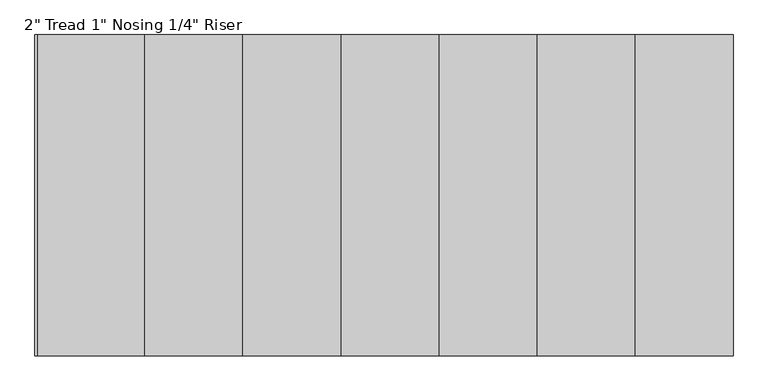
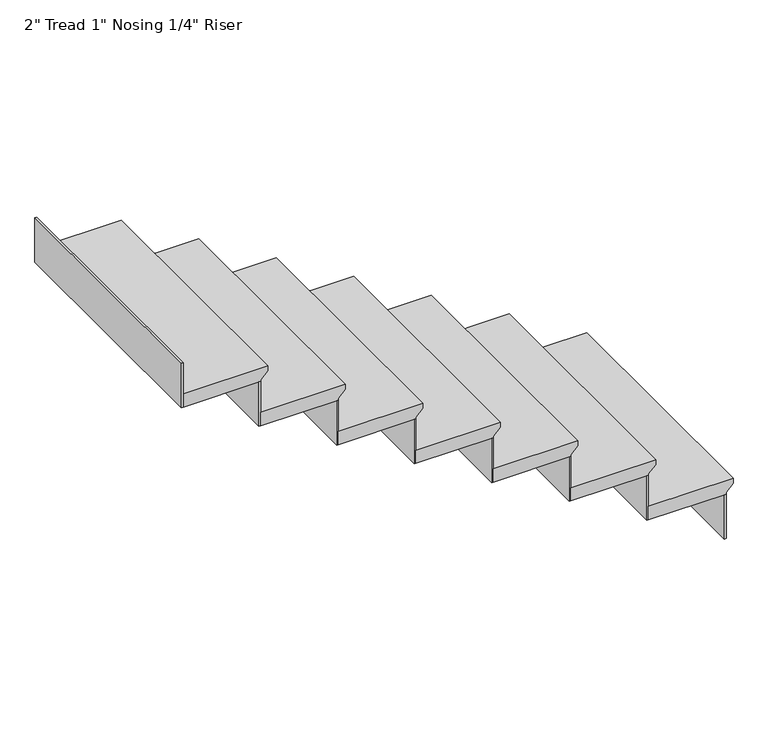
"""IFC4 building model written with IfcOpenShell, lengths in millimetres: stair flight geometry."""

from ifc_helpers import new_model, si_unit, frame, origin, place, context, project, spatial, polyline, outline, extrude, source, transform, mapped, element, save


def stair_flight_b96c5a2c(model_context):
    return source(origin(), model_context, "Body", "SweptSolid", [
        extrude(outline(polyline([(8077.2, 678.235938), (8077.2, 373.435938), (8026.4, 373.435938), (8026.4, 652.835938), (8032.75, 652.835938), (8058.15, 678.235938), (8077.2, 678.235938)])), frame((0.0, 1120.5857363, 0.0), z_axis=(0.0, 1.0, 0.0), x_axis=(0.0, 0.0, 1.0)), (0.0, 0.0, 1.0), 914.4),
        extrude(outline(polyline([(646.485938, 2034.9857363), (652.835938, 2034.9857363), (652.835938, 1120.5857363), (646.485938, 1120.5857363), (646.485938, 2034.9857363)])), frame((0.0, 0.0, 7857.0666667), z_axis=(0.0, 0.0, 1.0), x_axis=(1.0, 0.0, 0.0)), (0.0, 0.0, 1.0), 169.3333333),
        extrude(outline(polyline([(367.085938, 2034.9857363), (373.435938, 2034.9857363), (373.435938, 1120.5857363), (367.085938, 1120.5857363), (367.085938, 2034.9857363)])), frame((0.0, 0.0, 8026.4), z_axis=(0.0, 0.0, 1.0), x_axis=(1.0, 0.0, 0.0)), (0.0, 0.0, 1.0), 169.3333333),
        extrude(outline(polyline([(8246.5333333, 398.835938), (8246.5333333, 94.035938), (8195.7333333, 94.035938), (8195.7333333, 373.435938), (8202.0833333, 373.435938), (8227.4833333, 398.835938), (8246.5333333, 398.835938)])), frame((0.0, 1120.5857363, 0.0), z_axis=(0.0, 1.0, 0.0), x_axis=(0.0, 0.0, 1.0)), (0.0, 0.0, 1.0), 914.4),
        extrude(outline(polyline([(87.685938, 2034.9857363), (94.035938, 2034.9857363), (94.035938, 1120.5857363), (87.685938, 1120.5857363), (87.685938, 2034.9857363)])), frame((0.0, 0.0, 8195.7333333), z_axis=(0.0, 0.0, 1.0), x_axis=(1.0, 0.0, 0.0)), (0.0, 0.0, 1.0), 169.3333333),
        extrude(outline(polyline([(8415.8666667, 119.435938), (8415.8666667, -185.364062), (8365.0666667, -185.364062), (8365.0666667, 94.035938), (8371.4166667, 94.035938), (8396.8166667, 119.435938), (8415.8666667, 119.435938)])), frame((0.0, 1120.5857363, 0.0), z_axis=(0.0, 1.0, 0.0), x_axis=(0.0, 0.0, 1.0)), (0.0, 0.0, 1.0), 914.4),
        extrude(outline(polyline([(-191.714062, 2034.9857363), (-185.364062, 2034.9857363), (-185.364062, 1120.5857363), (-191.714062, 1120.5857363), (-191.714062, 2034.9857363)])), frame((0.0, 0.0, 8365.0666667), z_axis=(0.0, 0.0, 1.0), x_axis=(1.0, 0.0, 0.0)), (0.0, 0.0, 1.0), 169.3333333),
        extrude(outline(polyline([(8585.2, -159.964062), (8585.2, -464.764062), (8534.4, -464.764062), (8534.4, -185.364062), (8540.75, -185.364062), (8566.15, -159.964062), (8585.2, -159.964062)])), frame((0.0, 1120.5857363, 0.0), z_axis=(0.0, 1.0, 0.0), x_axis=(0.0, 0.0, 1.0)), (0.0, 0.0, 1.0), 914.4),
        extrude(outline(polyline([(-471.114062, 2034.9857363), (-464.764062, 2034.9857363), (-464.764062, 1120.5857363), (-471.114062, 1120.5857363), (-471.114062, 2034.9857363)])), frame((0.0, 0.0, 8534.4), z_axis=(0.0, 0.0, 1.0), x_axis=(1.0, 0.0, 0.0)), (0.0, 0.0, 1.0), 169.3333333),
        extrude(outline(polyline([(8754.5333333, -439.364062), (8754.5333333, -744.164062), (8703.7333333, -744.164062), (8703.7333333, -464.764062), (8710.0833333, -464.764062), (8735.4833333, -439.364062), (8754.5333333, -439.364062)])), frame((0.0, 1120.5857363, 0.0), z_axis=(0.0, 1.0, 0.0), x_axis=(0.0, 0.0, 1.0)), (0.0, 0.0, 1.0), 914.4),
        extrude(outline(polyline([(-750.514062, 2034.9857363), (-744.164062, 2034.9857363), (-744.164062, 1120.5857363), (-750.514062, 1120.5857363), (-750.514062, 2034.9857363)])), frame((0.0, 0.0, 8703.7333333), z_axis=(0.0, 0.0, 1.0), x_axis=(1.0, 0.0, 0.0)), (0.0, 0.0, 1.0), 169.3333333),
        extrude(outline(polyline([(8923.8666667, -718.764062), (8923.8666667, -1023.564062), (8873.0666667, -1023.564062), (8873.0666667, -744.164062), (8879.4166667, -744.164062), (8904.8166667, -718.764062), (8923.8666667, -718.764062)])), frame((0.0, 1120.5857363, 0.0), z_axis=(0.0, 1.0, 0.0), x_axis=(0.0, 0.0, 1.0)), (0.0, 0.0, 1.0), 914.4),
        extrude(outline(polyline([(-1029.914062, 2034.9857363), (-1023.564062, 2034.9857363), (-1023.564062, 1120.5857363), (-1029.914062, 1120.5857363), (-1029.914062, 2034.9857363)])), frame((0.0, 0.0, 8873.0666667), z_axis=(0.0, 0.0, 1.0), x_axis=(1.0, 0.0, 0.0)), (0.0, 0.0, 1.0), 169.3333333),
        extrude(outline(polyline([(-1309.314062, 2034.9857363), (-1302.964062, 2034.9857363), (-1302.964062, 1120.5857363), (-1309.314062, 1120.5857363), (-1309.314062, 2034.9857363)])), frame((0.0, 0.0, 9042.4), z_axis=(0.0, 0.0, 1.0), x_axis=(1.0, 0.0, 0.0)), (0.0, 0.0, 1.0), 169.3333333),
        extrude(outline(polyline([(9093.2, -998.164062), (9093.2, -1302.964062), (9042.4, -1302.964062), (9042.4, -1023.564062), (9048.75, -1023.564062), (9074.15, -998.164062), (9093.2, -998.164062)])), frame((0.0, 1120.5857363, 0.0), z_axis=(0.0, 1.0, 0.0), x_axis=(0.0, 0.0, 1.0)), (0.0, 0.0, 1.0), 914.4),
    ])


if __name__ == "__main__":
    model = new_model("IFC4")
    model_context = context("Model", 3, world=origin())
    ifc_project = project(units=[si_unit("LENGTHUNIT", "METRE", prefix="MILLI")], contexts=[model_context])
    site = spatial("IfcSite", under=ifc_project)
    building = spatial("IfcBuilding", under=site)
    placement = place(None, origin())
    stair_flight_shape = stair_flight_b96c5a2c(model_context)
    element("IfcStairFlight", 1, ObjectType="2\" Tread 1\" Nosing 1/4\" Riser", at=placement, inside=building, context=model_context, shape_type="MappedRepresentation", body=[
        mapped(stair_flight_shape, transform((0.0, 0.0, 0.0), x_axis=(1.0, 0.0, 0.0), y_axis=(0.0, 1.0, 0.0), z_axis=(0.0, 0.0, 1.0))),
    ])
    save(model, "model.ifc")

# Revit data of these elements
# Element 1 (IfcStairFlight, "2\" Tread 1\" Nosing 1/4\" Riser")
#   Materials on its faces: "BURGUNDY COLOUR"
# Materials
#   "BURGUNDY COLOUR": class "Generic", colour RGB 120 120 120, transparency 0, Cost = 0
